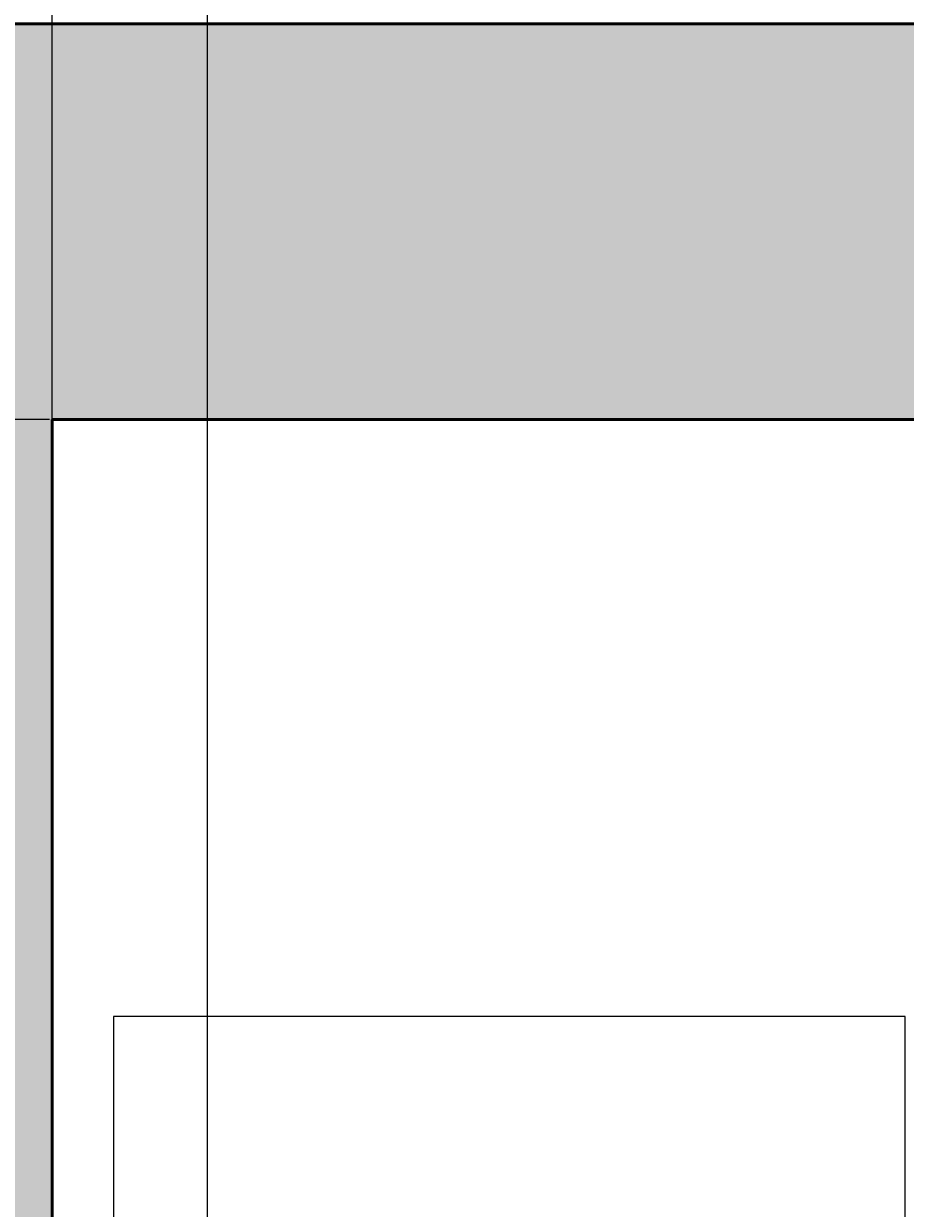
# Model space of a CAD drawing. Units: inches. Extents: x 2231 to 2461, y 2045 to 2455.
# Tile 75 of 95: x 2258 to 2278, y 2409 to 2436. Entities that reach past the tile are written whole.
import ezdxf

# ---------------------------------------------------------------- set-up
doc = ezdxf.new("R2010")
doc.units = ezdxf.units.IN
for name, color, linetype, lineweight in [('A-ANNO-DIMS', 2, 'Continuous', 18), ('A-FURN', 9, 'Continuous', 18), ('A-WALL', 7, 'Continuous', 50)]:
    doc.layers.add(name, color=color, linetype=linetype, lineweight=lineweight)
doc.layers.add('A-WALL-PATT', color=18, linetype='Continuous', lineweight=13, true_color=0x000000)
doc.styles.get("Standard").update_dxf_attribs({"font": 'arial.ttf'})
doc.dimstyles.get("Standard").update_dxf_attribs({"dimtxt": 0.18, "dimasz": 0.18, "dimexe": 0.18, "dimexo": 0.0625, "dimgap": 0.09, "dimtad": 0, "dimtih": 1, "dimtoh": 1, "dimdec": 4, "dimzin": 0, "dimdsep": 46, "dimtxsty": 'Standard', "dimcen": 0.09, "dimadec": 0, "dimazin": 0, "dimtfac": 1, "dimtdec": 4, "dimtofl": 0, "dimtmove": 0, "dimatfit": 3, "dimfxl": 1, "dimtolj": 1, "dimtzin": 0, "dimarcsym": 0})

# ---------------------------------------------------------------- blocks, each defined once
blk = doc.blocks.new('NIGHTSTAND-18IN')
blk.add_lwpolyline([(0, 0), (18, 0), (18, 18), (0, 18)], close=True)
blk = doc.blocks.new('*D35')
at = {"layer": 'A-ANNO-DIMS', "color": 0, "lineweight": -2, "transparency": 16777216}
for p, q in [((2258.794, 2426.895), (2258.794, 2454.645)), ((2368.794, 2426.895), (2368.794, 2454.645)), ((2258.974, 2454.465), (2313.513, 2454.465)), ((2368.614, 2454.465), (2314.074, 2454.465))]:
    blk.add_line(p, q, dxfattribs=at)
at = {"layer": 'A-ANNO-DIMS', "color": 0, "transparency": 16777216}
for points in [[(2258.974, 2454.495), (2258.974, 2454.435), (2258.794, 2454.465)], [(2368.614, 2454.495), (2368.614, 2454.435), (2368.794, 2454.465)]]:
    blk.add_solid(points, dxfattribs=at)
at = {"layer": 'Defpoints', "color": 0, "transparency": 16777216}
for p in [(2368.794, 2454.465), (2258.794, 2426.833), (2368.794, 2426.833)]:
    blk.add_point(p, dxfattribs=at)
at = {"layer": 'A-ANNO-DIMS', "color": 0, "transparency": 16777216, "insert": (2313.794, 2454.465), "char_height": 0.18, "attachment_point": 5}
blk.add_mtext('\\A1;110', dxfattribs=at)
blk = doc.blocks.new('*D37')
at = {"layer": 'A-ANNO-DIMS', "color": 0, "lineweight": -2, "transparency": 16777216}
for p, q in [((2258.731, 2426.833), (2230.981, 2426.833)), ((2231.161, 2426.653), (2231.161, 2367.015)), ((2231.161, 2307.013), (2231.161, 2366.651)), ((2258.731, 2306.833), (2230.981, 2306.833))]:
    blk.add_line(p, q, dxfattribs=at)
at = {"layer": 'A-ANNO-DIMS', "color": 0, "transparency": 16777216}
for points in [[(2231.131, 2426.653), (2231.191, 2426.653), (2231.161, 2426.833)], [(2231.131, 2307.013), (2231.191, 2307.013), (2231.161, 2306.833)]]:
    blk.add_solid(points, dxfattribs=at)
at = {"layer": 'Defpoints', "color": 0, "transparency": 16777216}
for p in [(2231.161, 2426.833), (2258.794, 2426.833), (2258.794, 2306.833)]:
    blk.add_point(p, dxfattribs=at)
at = {"layer": 'A-ANNO-DIMS', "color": 0, "transparency": 16777216, "insert": (2231.161, 2366.833), "char_height": 0.18, "attachment_point": 5}
blk.add_mtext('\\A1;120', dxfattribs=at)
blk = doc.blocks.new('*D47')
at = {"layer": 'A-ANNO-DIMS', "color": 0, "lineweight": -2, "transparency": 16777216}
for p, q in [((2258.794, 2182.895), (2258.794, 2454.645)), ((2294.794, 2182.895), (2294.794, 2454.645)), ((2258.974, 2454.465), (2276.575, 2454.465)), ((2294.614, 2454.465), (2277.012, 2454.465))]:
    blk.add_line(p, q, dxfattribs=at)
at = {"layer": 'A-ANNO-DIMS', "color": 0, "transparency": 16777216}
for points in [[(2258.974, 2454.495), (2258.974, 2454.435), (2258.794, 2454.465)], [(2294.614, 2454.495), (2294.614, 2454.435), (2294.794, 2454.465)]]:
    blk.add_solid(points, dxfattribs=at)
at = {"layer": 'Defpoints', "color": 0, "transparency": 16777216}
for p in [(2294.794, 2454.465), (2258.794, 2182.833), (2294.794, 2182.833)]:
    blk.add_point(p, dxfattribs=at)
at = {"layer": 'A-ANNO-DIMS', "color": 0, "transparency": 16777216, "insert": (2276.794, 2454.465), "char_height": 0.18, "attachment_point": 5}
blk.add_mtext('\\A1;36', dxfattribs=at)
blk = doc.blocks.new('*D62')
at = {"layer": 'A-ANNO-DIMS', "color": 0, "lineweight": -2, "transparency": 16777216}
for p, q in [((2262.321, 2255.176), (2262.321, 2454.645)), ((2292.321, 2253.176), (2292.321, 2454.645)), ((2262.501, 2454.465), (2277.102, 2454.465)), ((2292.141, 2454.465), (2277.539, 2454.465))]:
    blk.add_line(p, q, dxfattribs=at)
at = {"layer": 'A-ANNO-DIMS', "color": 0, "transparency": 16777216}
for points in [[(2262.501, 2454.495), (2262.501, 2454.435), (2262.321, 2454.465)], [(2292.141, 2454.495), (2292.141, 2454.435), (2292.321, 2454.465)]]:
    blk.add_solid(points, dxfattribs=at)
at = {"layer": 'Defpoints', "color": 0, "transparency": 16777216}
for p in [(2292.321, 2454.465), (2262.321, 2255.114), (2292.321, 2253.114)]:
    blk.add_point(p, dxfattribs=at)
at = {"layer": 'A-ANNO-DIMS', "color": 0, "transparency": 16777216, "insert": (2277.321, 2454.465), "char_height": 0.18, "attachment_point": 5}
blk.add_mtext('\\A1;30', dxfattribs=at)

msp = doc.modelspace()

# ---------------------------------------------------------------- hatches: boundary and pattern name
at = {"layer": 'A-WALL-PATT'}
h = msp.add_hatch(color=256, dxfattribs=at)
h.dxf.hatch_style = 1
h.paths.add_polyline_path([(2441.7935, 2269.1535), (2432.7935, 2269.1535), (2432.7935, 2186.8328), (2396.7935, 2186.8328), (2396.7935, 2286.8328), (2394.7935, 2286.8328), (2394.7935, 2186.8328), (2334.7935, 2186.8328), (2334.7935, 2182.8328), (2432.7935, 2182.8328), (2432.7935, 2072.8328), (2416.6639, 2072.8328), (2416.6639, 2063.8328), (2441.7935, 2063.8328)])
h.paths.add_polyline_path([(2368.6639, 2072.8328), (2367.04, 2072.8328), (2330.7942, 2072.8328), (2330.7397, 2063.8328), (2368.6639, 2063.8328)])
h.paths.add_polyline_path([(2300.7392, 2068.3328), (2300.7392, 2072.8328), (2298.7935, 2072.8328), (2294.7935, 2072.8328), (2258.7935, 2072.8328), (2258.7935, 2120.8328), (2294.7935, 2120.8328), (2298.7935, 2120.8328), (2298.7935, 2128.8328), (2294.7935, 2128.8328), (2294.7935, 2124.8328), (2258.7935, 2124.8328), (2258.7935, 2182.8328), (2294.7935, 2182.8328), (2294.7935, 2174.8328), (2298.7935, 2174.8328), (2298.7935, 2182.8328), (2304.7935, 2182.8328), (2304.7935, 2186.8328), (2258.7935, 2186.8328), (2258.7935, 2221.999), (2249.7935, 2221.999), (2249.7935, 2063.8328), (2300.7392, 2063.8328)])
h.paths.add_polyline_path([(2391.9338, 2435.8328), (2333.82, 2435.8328), (2333.82, 2426.8328), (2368.7935, 2426.8328), (2368.7935, 2374.9508), (2368.7935, 2370.8328), (2372.3935, 2370.8328), (2372.7935, 2370.8328), (2372.7935, 2426.8328), (2391.9338, 2426.8328)])
h.paths.add_polyline_path([(2441.7935, 2435.8328), (2415.9338, 2435.8328), (2415.9338, 2426.8328), (2432.7935, 2426.8328), (2432.7935, 2334.8328), (2372.7935, 2334.8328), (2372.7935, 2346.8328), (2368.7935, 2346.8328), (2368.7935, 2306.8328), (2360.7935, 2306.8328), (2360.7935, 2302.8328), (2368.7935, 2302.8328), (2372.7935, 2302.8328), (2372.7935, 2330.8328), (2432.7935, 2330.8328), (2432.7935, 2317.1535), (2441.7935, 2317.1535)])
h.paths.add_polyline_path([(2285.82, 2435.8328), (2249.7935, 2435.8328), (2249.7935, 2269.999), (2258.7935, 2269.999), (2258.7935, 2302.8328), (2318.8168, 2302.8328), (2330.7935, 2302.8328), (2330.7935, 2306.8328), (2258.7935, 2306.8328), (2258.7935, 2426.8328), (2285.82, 2426.8328)])

# ---------------------------------------------------------------- linework, layer by layer
at = {"layer": 'A-WALL'}
for p, q in [((2258.7935, 2426.8328), (2368.7935, 2426.8328)), ((2258.7935, 2306.8328), (2258.7935, 2426.8328))]:
    msp.add_line(p, q, dxfattribs=at)
msp.add_lwpolyline([(2300.7392, 2063.8328), (2249.7935, 2063.8328), (2249.7935, 2435.8328), (2441.7935, 2435.8328), (2441.7935, 2063.8328), (2330.7397, 2063.8328)], dxfattribs=at)

# ---------------------------------------------------------------- block references
at = {"layer": 'A-FURN'}
msp.add_blockref('NIGHTSTAND-18IN', (2260.188, 2395.253), dxfattribs=at)

# ---------------------------------------------------------------- dimensions: what is measured, and where the dimension line sits
at = {"layer": 'A-ANNO-DIMS'}
for base, p1, p2, picture, middle in [((2368.7935, 2454.4653), (2258.7935, 2426.8328), (2368.7935, 2426.8328), '*D35', (2313.7935, 2454.4653)), ((2294.7935, 2454.4653), (2258.7935, 2182.8328), (2294.7935, 2182.8328), '*D47', (2276.7935, 2454.4653)), ((2292.3207, 2454.4653), (2262.3207, 2255.1137), (2292.3207, 2253.1137), '*D62', (2277.3207, 2454.4653))]:
    dim = msp.add_linear_dim(base=base, p1=p1, p2=p2, dimstyle='Standard', override={"dimdec": 0, "dimlfac": 1, "dimrnd": 0, "dimzin": 0, "dimdsep": 46, "dimlunit": 2}, dxfattribs=at)
    dim.commit()
    dim.dimension.update_dxf_attribs({"geometry": picture, "text_midpoint": middle})
dim = msp.add_linear_dim(base=(2231.161, 2426.8328), p1=(2258.7935, 2306.8328), p2=(2258.7935, 2426.8328), angle=90, dimstyle='Standard', override={"dimdec": 0, "dimlfac": 1, "dimrnd": 0, "dimzin": 0, "dimdsep": 46, "dimlunit": 2}, dxfattribs=at)
dim.commit()
dim.dimension.update_dxf_attribs({"geometry": '*D37', "text_midpoint": (2231.161, 2366.8328)})

doc.saveas('drawing.dxf')
